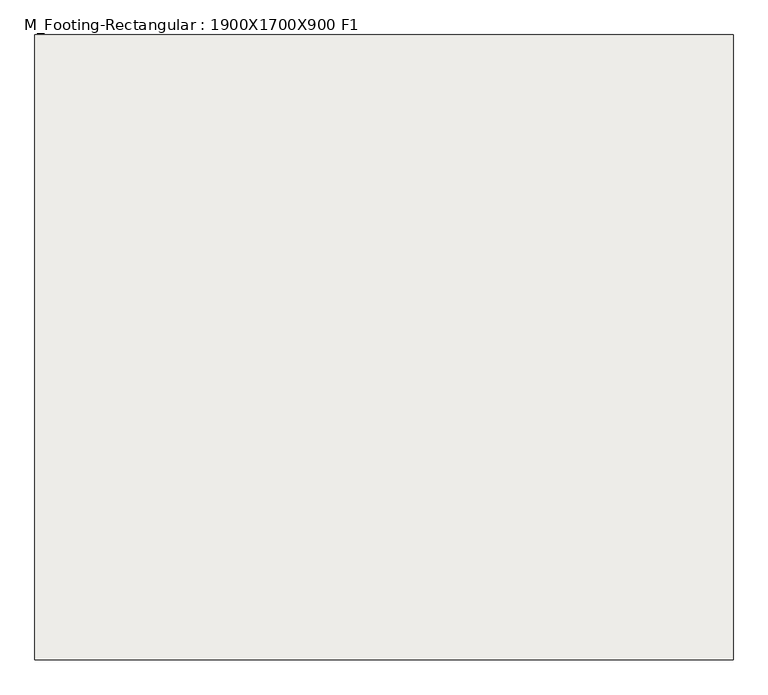
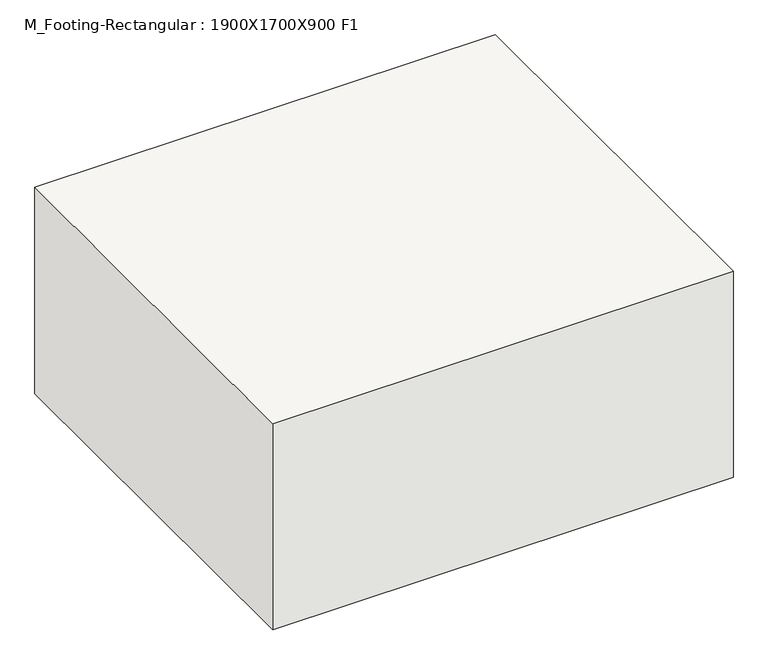
"""IFC4 building model written with IfcOpenShell, lengths in millimetres: slab geometry, M_Footing-Rectangular : 1900X1700X900 F1."""

from ifc_helpers import new_model, si_unit, frame, origin, place, context, project, spatial, polyline, outline, extrude, source, transform, mapped, element, save


def m_footing_rectangular_1900x1700x900_f1_617558a1(model_context):
    return source(origin(), model_context, "Body", "SweptSolid", [
        extrude(outline(polyline([(950.0, 850.0), (950.0, -850.0), (-950.0, -850.0), (-950.0, 850.0), (950.0, 850.0)])), frame((0.0, 0.0, -900.0), z_axis=(0.0, 0.0, 1.0), x_axis=(1.0, 0.0, 0.0)), (0.0, 0.0, 1.0), 900.0),
    ])


if __name__ == "__main__":
    model = new_model("IFC4")
    model_context = context("Model", 3, world=origin())
    ifc_project = project(units=[si_unit("LENGTHUNIT", "METRE", prefix="MILLI")], contexts=[model_context])
    site = spatial("IfcSite", under=ifc_project)
    building = spatial("IfcBuilding", under=site)
    placement = place(None, origin())
    m_footing_rectangular_1900x1700x900_f1_shape = m_footing_rectangular_1900x1700x900_f1_617558a1(model_context)
    element("IfcSlab", 1, ObjectType="M_Footing-Rectangular : 1900X1700X900 F1", at=placement, inside=building, context=model_context, shape_type="MappedRepresentation", body=[
        mapped(m_footing_rectangular_1900x1700x900_f1_shape, transform((0.0, 0.0, 0.0), x_axis=(1.0, 0.0, 0.0), y_axis=(0.0, 1.0, 0.0), z_axis=(0.0, 0.0, 1.0))),
    ])
    save(model, "model.ifc")

# Revit data of these elements
# Type "M_Footing-Rectangular : 1900X1700X900 F1"
#   Width = 1900 mm
#   Length = 1700 mm
#   Foundation Thickness = 900 mm
#   Structural Material [instance default] = Concrete, Cast-in-Place gray
#   Assembly Code = ""
# Element 1 (IfcSlab, "M_Footing-Rectangular : 1900X1700X900 F1")
#   Structural Material = Concrete, Cast In Situ
#   Materials on its faces: "Concrete, Cast In Situ"
# Materials
#   "Concrete, Cast-in-Place gray": class "Concrete", colour RGB 192 192 192, transparency 0, Description = "Cast-in-place concrete", Cost = 0
#   "Concrete, Cast In Situ": class "Concrete", colour RGB 192 192 192, transparency 0, Description = "physical material", Cost = 0
